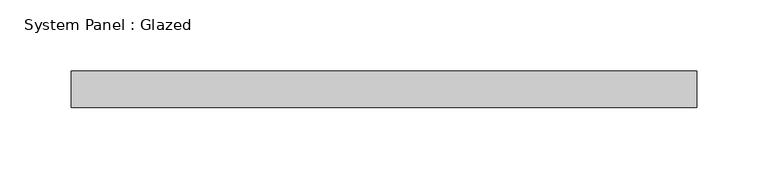
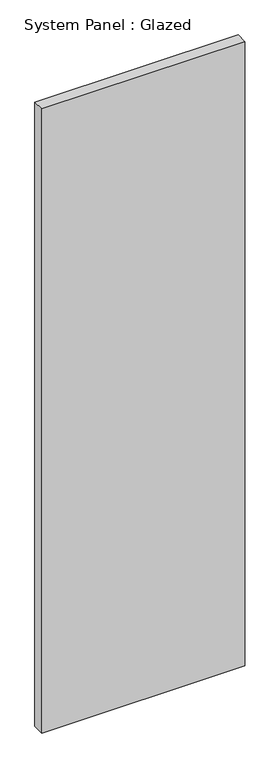
"""IFC4 building model written with IfcOpenShell, lengths in millimetres: plate geometry, System Panel : Glazed."""

from ifc_helpers import new_model, si_unit, origin, origin_with_axes, place, context, project, spatial, polyline, outline, extrude, source, transform, mapped, element, save


def system_panel_glazed_78e3b77e(model_context):
    return source(origin(), model_context, "Body", "SweptSolid", [
        extrude(outline(polyline([(219.075, 19.05), (-219.075, 19.05), (-219.075, 44.45), (219.075, 44.45), (219.075, 19.05)])), origin_with_axes(), (0.0, 0.0, 1.0), 1423.2845828),
    ])


if __name__ == "__main__":
    model = new_model("IFC4")
    model_context = context("Model", 3, world=origin())
    ifc_project = project(units=[si_unit("LENGTHUNIT", "METRE", prefix="MILLI")], contexts=[model_context])
    site = spatial("IfcSite", under=ifc_project)
    building = spatial("IfcBuilding", under=site)
    placement = place(None, origin())
    system_panel_glazed_shape = system_panel_glazed_78e3b77e(model_context)
    element("IfcPlate", 1, ObjectType="System Panel : Glazed", at=placement, inside=building, context=model_context, shape_type="MappedRepresentation", body=[
        mapped(system_panel_glazed_shape, transform((0.0, 0.0, 0.0), x_axis=(1.0, 0.0, 0.0), y_axis=(0.0, 1.0, 0.0), z_axis=(0.0, 0.0, 1.0))),
    ])
    save(model, "model.ifc")

# Revit data of these elements
# Type "System Panel : Glazed"
#   Construction Type Id = "GSP4R"
#   Analytic Construction = "1/8 in Pilkington single glazing"
#   Visual Light Transmittance = 0.9
#   Solar Heat Gain Coefficient = 0.86
#   Heat Transfer Coefficient (U) = 1.18115 BTU/(h·ft²·°F)
#   Define Thermal Properties by = 1
# Element 1 (IfcPlate, "System Panel : Glazed")
#   Materials on its faces: "Glass"
# Materials
#   "Glass": class "Glass", colour RGB 0 128 192, transparency 0.75, Description = "Soda Lime Glass", Cost = 0
